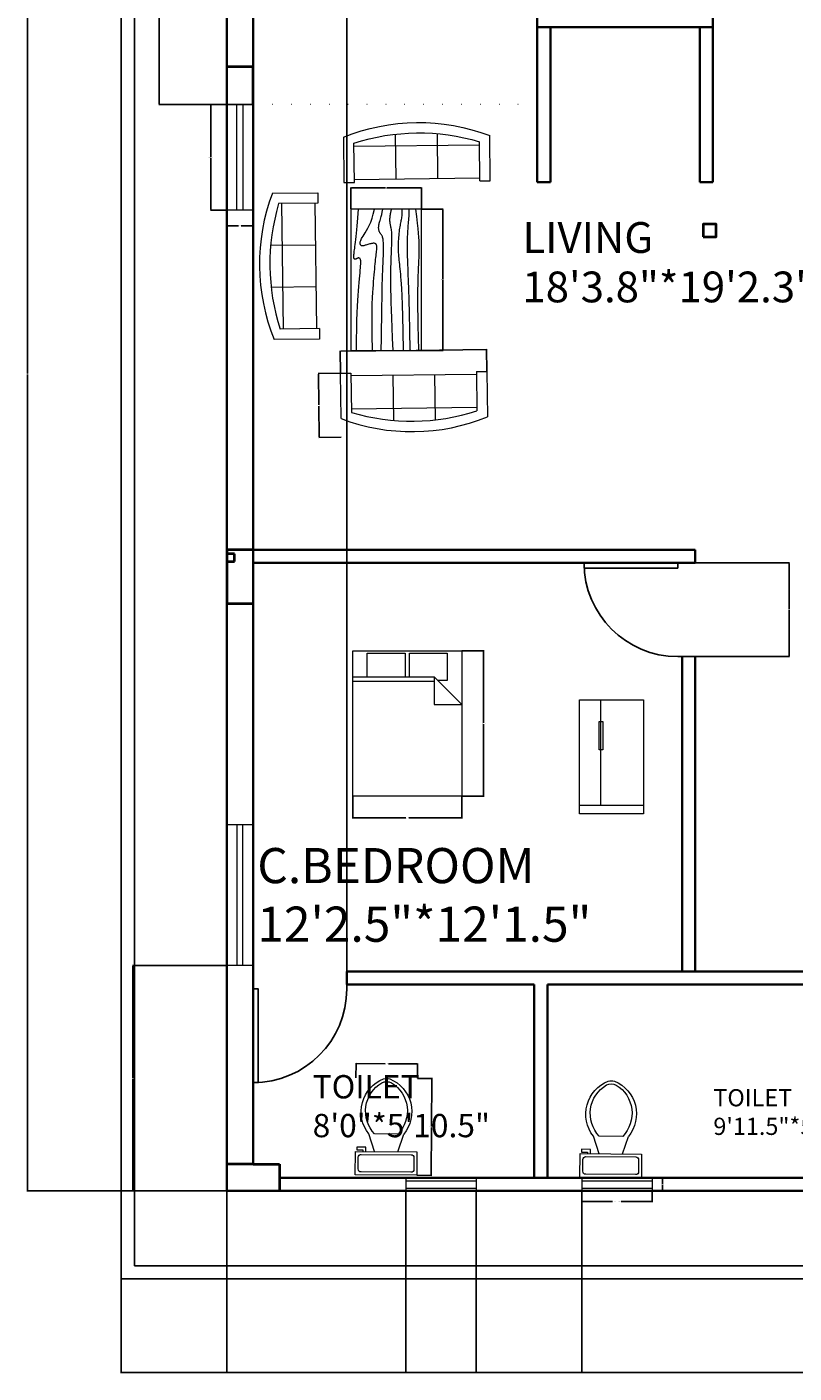
# Model space of a CAD drawing. Units: inches. Extents: x -1085 to 1941, y 1514 to 2348.
# Tile 7 of 9: x 1397 to 1659, y 1514 to 1974. Entities that reach past the tile are written whole.
import ezdxf

# ---------------------------------------------------------------- set-up
doc = ezdxf.new("R2010")
doc.units = ezdxf.units.IN
doc.linetypes.add('DOT', pattern=[6.35, 0, -6.35])
for name, color, linetype, lineweight in [('A-ANNO-DIMS', 2, 'Continuous', 18), ('A-AREA-IDEN', 7, 'Continuous', 25), ('A-COLS', 7, 'Continuous', 40), ('A-DOOR', 4, 'Continuous', 25), ('A-EQPM', 9, 'Continuous', 18), ('A-FLOR-FIXT', 9, 'Continuous', 18), ('A-GLAZ', 180, 'Continuous', 18), ('A-WALL', 7, 'Continuous', 35), ('A-WALL-OVHD', 8, 'DOT', 18), ('C-PROP', 8, 'Continuous', 25), ('FOUNITR-URE', 2, 'Continuous', 18)]:
    doc.layers.add(name, color=color, linetype=linetype, lineweight=lineweight)
doc.styles.get("Standard").update_dxf_attribs({"font": 'arial.ttf'})
doc.dimstyles.get("Standard").update_dxf_attribs({"dimtxt": 0.18, "dimasz": 0.18, "dimexe": 0.18, "dimexo": 0.0625, "dimgap": 0.09, "dimtad": 0, "dimtih": 1, "dimtoh": 1, "dimdec": 4, "dimzin": 0, "dimdsep": 46, "dimtxsty": 'Standard', "dimcen": 0.09, "dimadec": 0, "dimazin": 0, "dimtfac": 1, "dimtdec": 4, "dimtofl": 0, "dimtmove": 0, "dimatfit": 3, "dimfxl": 1, "dimtolj": 1, "dimtzin": 0, "dimarcsym": 0})

# ---------------------------------------------------------------- blocks, each defined once
blk = doc.blocks.new('*U3')
for p, q in [((0, 0), (0, -6)), ((32, 0), (32, -6))]:
    blk.add_line(p, q)
blk.add_lwpolyline([(0, 0), (0, 32), (1.75, 32), (1.75, 0)], close=True)
blk.add_arc((0, 0), 32, 0, 90)
blk = doc.blocks.new('Bed - Queen')
for p, q in [((0, -80.00003), (0, 0)), ((0, 0), (59.99999, 0)), ((59.99999, 0), (59.99999, -80.00003)), ((7.99999, -1.2), (28.79998, -1.2)), ((7.99999, -14.4), (7.99999, -1.2)), ((28.79998, -1.2), (28.79998, -14.4)), ((31.19999, -1.2), (51.99999, -1.2)), ((31.19999, -14.4), (31.19999, -1.2)), ((51.99999, -1.2), (51.99999, -16.4)), ((0, -14.4), (44.8, -14.4)), ((59.99999, -29.6), (44.8, -14.4)), ((44.8, -14.4), (44.8, -29.6)), ((44.8, -16.8), (0, -16.8)), ((51.99999, -16.4), (46.79936, -16.4)), ((44.8, -29.6), (59.99999, -29.6)), ((59.99999, -80.00003), (0, -80.00003))]:
    blk.add_line(p, q)
blk = doc.blocks.new('Refrigerator-2 door - 36 in front')
for p, q in [((12, 5), (12, 64)), ((0, 5), (36, 5))]:
    blk.add_line(p, q)
for points in [[(0, 0), (0, 64), (36, 64), (36, 0)], [(11, 36), (11, 52), (13, 52), (13, 36)]]:
    blk.add_lwpolyline(points, close=True)
blk = doc.blocks.new('Toilet - top')
for p, q in [((9.5, -6), (9.5, -2)), ((-10, -8.5), (-8, -8.5)), ((-10, -9.5), (-10, -8.5)), ((-8, -8.5), (-8, -8)), ((-7, -8), (-7, -9.5)), ((-4, -8), (-6, -14)), ((4, -8), (6, -14)), ((-7, -9.5), (-10, -9.5)), ((4, -14), (-4, -14))]:
    blk.add_line(p, q)
blk.add_lwpolyline([(10.5, -8), (10.5, 0), (-10.5, 0), (-10.5, -8)], close=True)
for points in [[(-9.5, -2), (-9.5, -6)], [(8.5, -1), (-8.5, -1)], [(-8.5, -7), (8.5, -7)]]:
    blk.add_lwpolyline(points)
for centre, radius, start, end in [((-8.62, -1.88), 0.884, 81.8699, 188.1301), ((8.62, -1.88), 0.884, 351.8699, 98.1301), ((-8.62, -6.12), 0.884, 171.8699, 278.1301), ((8.62, -6.12), 0.884, 261.8699, 8.1301), ((3.52, -21.58), 12.17, 141.4691, 247.9714), ((4.2, -21.82), 11.33, 136.3677, 238.9468), ((-3.52, -21.58), 12.17, 292.0284, 38.5307), ((-4.2, -21.82), 11.33, 301.053, 43.6321), ((0, -27.88), 4, 245.7318, 294.2682), ((0, -29), 4, 254.8605, 285.1395)]:
    blk.add_arc(centre, radius, start, end)
blk = doc.blocks.new('Table - Rectangular Woodgrain 60 x 30 in.')
for p, q in [((0, 0), (0, -30)), ((60, 0), (0, 0)), ((60, -30), (60, 0)), ((0, -30), (60, -30))]:
    blk.add_line(p, q)
for points in [[(0, -2.4), (4.8155, -2.418), (9.0302, -2.4688), (12.709, -2.5477), (15.9167, -2.65), (18.7181, -2.7711), (21.1781, -2.9063), (23.3616, -3.0508), (25.3333, -3.2), (27.1477, -3.3495), (28.8172, -3.4958), (30.3437, -3.636), (31.7291, -3.7667), (32.9756, -3.8849), (34.0849, -3.9875), (35.059, -4.0714), (35.9, -4.1334), (36.6114, -4.1711), (37.2041, -4.1854), (37.6906, -4.1779), (38.0833, -4.15), (38.3948, -4.1034), (38.6375, -4.0396), (38.8239, -3.9602), (38.9666, -3.8667), (39.0764, -3.7608), (39.1573, -3.6448), (39.2116, -3.521), (39.2416, -3.3917), (39.2498, -3.2593), (39.2385, -3.1261), (39.21, -2.9944), (39.1666, -2.8667), (39.111, -2.7447), (39.0468, -2.6281), (38.978, -2.5163), (38.9083, -2.4083), (38.8418, -2.3035), (38.7823, -2.201), (38.7337, -2.1001), (38.7, -2), (38.6844, -1.9003), (38.6875, -1.8021), (38.7094, -1.707), (38.75, -1.6167), (38.8094, -1.5326), (38.8875, -1.4563), (38.9844, -1.3893), (39.1, -1.3333), (39.2351, -1.2896), (39.3937, -1.2583), (39.5804, -1.2396), (39.8, -1.2333), (40.057, -1.2396), (40.3562, -1.2583), (40.7023, -1.2896), (41.1, -1.3333), (41.5547, -1.3895), (42.0755, -1.4573), (42.6721, -1.5361), (43.3542, -1.625), (44.1316, -1.7233), (45.014, -1.8302), (46.0114, -1.9449), (47.1333, -2.0667), (48.3862, -2.1947), (49.7625, -2.3281), (51.2513, -2.4663), (52.8416, -2.6083), (54.5226, -2.7535), (56.2833, -2.9011), (58.1127, -3.0501), (60, -3.2)], [(0, -9.2), (6.5759, -9.0858), (11.9385, -9.0365), (16.2527, -9.0418), (19.6833, -9.0917), (22.3952, -9.1759), (24.5531, -9.2844), (26.322, -9.4069), (27.8666, -9.5333), (29.3241, -9.6553), (30.7203, -9.7719), (32.0532, -9.8837), (33.3208, -9.9917), (34.5213, -10.0965), (35.6526, -10.199), (36.7128, -10.2999), (37.7, -10.4), (38.6129, -10.4996), (39.4531, -10.5969), (40.223, -10.6895), (40.925, -10.775), (41.5613, -10.8512), (42.1344, -10.9156), (42.6465, -10.966), (43.1, -11), (43.4976, -11.0158), (43.8437, -11.0136), (44.143, -10.9942), (44.4, -10.9583), (44.6195, -10.9069), (44.8062, -10.8406), (44.9648, -10.7603), (45.1, -10.6667), (45.2155, -10.5598), (45.3114, -10.4365), (45.3871, -10.2929), (45.4416, -10.125), (45.4743, -9.929), (45.4844, -9.7011), (45.4709, -9.4371), (45.4333, -9.1333), (45.3716, -8.7883), (45.2896, -8.4104), (45.1919, -8.0107), (45.0833, -7.6), (44.9685, -7.1893), (44.8521, -6.7896), (44.7388, -6.4117), (44.6333, -6.0667), (44.54, -5.7628), (44.4614, -5.4979), (44.4001, -5.2675), (44.3583, -5.0667), (44.3384, -4.8909), (44.3427, -4.7354), (44.3736, -4.5956), (44.4333, -4.4667), (44.5236, -4.3453), (44.6427, -4.2333), (44.7884, -4.1339), (44.9583, -4.05), (45.1501, -3.9849), (45.3614, -3.9417), (45.59, -3.9234), (45.8333, -3.9333), (46.0915, -3.9749), (46.3734, -4.0531), (46.6906, -4.1736), (47.0542, -4.3417), (47.4756, -4.5629), (47.9661, -4.8427), (48.5372, -5.1866), (49.2, -5.6), (49.9676, -6.0844), (50.8594, -6.625), (51.8965, -7.2031), (53.1, -7.8), (54.491, -8.3969), (56.0906, -8.975), (57.9199, -9.5156), (60, -10)], [(0, -12.8), (5.1847, -12.9322), (9.6213, -13.0323), (13.3963, -13.1059), (16.5958, -13.1583), (19.3063, -13.1952), (21.614, -13.2219), (23.6054, -13.2439), (25.3666, -13.2667), (26.9728, -13.2947), (28.4531, -13.3281), (29.8256, -13.3663), (31.1083, -13.4083), (32.3191, -13.4535), (33.476, -13.501), (34.597, -13.5501), (35.7, -13.6), (36.7984, -13.6497), (37.8875, -13.6979), (38.9578, -13.743), (40, -13.7833), (41.0047, -13.8174), (41.9625, -13.8438), (42.864, -13.8607), (43.7, -13.8667), (44.4631, -13.8604), (45.1552, -13.8417), (45.7801, -13.8104), (46.3416, -13.7667), (46.8439, -13.7104), (47.2906, -13.6417), (47.6858, -13.5604), (48.0333, -13.4667), (48.3375, -13.3608), (48.6042, -13.2448), (48.8396, -13.121), (49.05, -12.9917), (49.2417, -12.8593), (49.4208, -12.7261), (49.5937, -12.5944), (49.7667, -12.4667), (49.9452, -12.3451), (50.1323, -12.2313), (50.3303, -12.1268), (50.5416, -12.0333), (50.7686, -11.9524), (51.0135, -11.8854), (51.2788, -11.8341), (51.5666, -11.8), (51.8785, -11.7843), (52.2116, -11.7865), (52.562, -11.8059), (52.926, -11.8417), (53.2998, -11.8931), (53.6795, -11.9594), (54.0614, -12.0397), (54.4416, -12.1333), (54.8223, -12.2401), (55.2293, -12.3625), (55.6942, -12.5037), (56.2489, -12.6667), (56.9251, -12.8547), (57.7545, -13.0708), (58.7689, -13.3182), (60, -13.6)], [(0, -18), (5.124, -17.7273), (9.6609, -17.5057), (13.6705, -17.3303), (17.2125, -17.1958), (20.3467, -17.0973), (23.1328, -17.0297), (25.6307, -16.9878), (27.9, -16.9667), (29.9928, -16.9617), (31.9302, -16.9703), (33.7254, -16.9907), (35.3917, -17.0208), (36.9423, -17.0588), (38.3906, -17.1026), (39.7499, -17.1503), (41.0333, -17.2), (42.2519, -17.2496), (43.4073, -17.2969), (44.4986, -17.3395), (45.525, -17.375), (46.4858, -17.4012), (47.3802, -17.4156), (48.2074, -17.416), (48.9667, -17.4), (49.6583, -17.3662), (50.2872, -17.3167), (50.8595, -17.2547), (51.3812, -17.1833), (51.8584, -17.1057), (52.2971, -17.025), (52.7034, -16.9443), (53.0833, -16.8667), (53.443, -16.7951), (53.789, -16.7313), (54.128, -16.6768), (54.4666, -16.6334), (54.8115, -16.6024), (55.1693, -16.5854), (55.5465, -16.5841), (55.95, -16.6), (56.3828, -16.6337), (56.8346, -16.6823), (57.2915, -16.7418), (57.7396, -16.8084), (58.165, -16.878), (58.5539, -16.9469), (58.8924, -17.0111), (59.1666, -17.0667), (59.3679, -17.1107), (59.5078, -17.1438), (59.6032, -17.1675), (59.6708, -17.1833), (59.7275, -17.193), (59.7901, -17.1979), (59.8753, -17.1998), (60, -17.2)], [(0, -22.4), (8.0098, -22.2501), (14.4094, -22.1011), (19.4168, -21.9535), (23.25, -21.8083), (26.1269, -21.6663), (28.2656, -21.5281), (29.884, -21.3947), (31.2, -21.2667), (32.3967, -21.1448), (33.5172, -21.0292), (34.5697, -20.9198), (35.5625, -20.8167), (36.5037, -20.7198), (37.4015, -20.6292), (38.2642, -20.5448), (39.1, -20.4667), (39.9164, -20.3951), (40.7187, -20.3313), (41.5117, -20.2768), (42.3, -20.2333), (43.0883, -20.2024), (43.8812, -20.1854), (44.6836, -20.1841), (45.5, -20.2), (46.3328, -20.234), (47.1747, -20.2844), (48.0163, -20.3488), (48.8479, -20.425), (49.66, -20.5106), (50.4429, -20.6031), (51.1872, -20.7004), (51.8833, -20.8), (52.5246, -20.8999), (53.1166, -20.9995), (53.6681, -21.0983), (54.1875, -21.1958), (54.6834, -21.2919), (55.1646, -21.3859), (55.6394, -21.4777), (56.1167, -21.5667), (56.6028, -21.6515), (57.0961, -21.7266), (57.5929, -21.7852), (58.0896, -21.8208), (58.5823, -21.8268), (59.0674, -21.7964), (59.5412, -21.723), (60, -21.6)], [(0, -25.2), (8.6355, -25.0504), (15.7026, -24.9031), (21.4049, -24.7606), (25.9458, -24.625), (29.529, -24.4988), (32.3578, -24.3844), (34.6359, -24.284), (36.5667, -24.2), (38.3213, -24.1341), (39.9417, -24.0854), (41.437, -24.0523), (42.8167, -24.0333), (44.0901, -24.0268), (45.2667, -24.0313), (46.3557, -24.0451), (47.3667, -24.0667), (48.309, -24.0947), (49.1928, -24.1287), (50.0284, -24.168), (50.826, -24.2125), (51.5959, -24.2617), (52.3483, -24.3151), (53.0935, -24.3725), (53.8417, -24.4334), (54.6009, -24.497), (55.3699, -24.561), (56.1454, -24.6226), (56.9239, -24.6792), (57.7021, -24.7279), (58.4764, -24.7662), (59.2435, -24.7911), (60, -24.8)], [(0, -28.8), (5.6867, -28.6681), (10.45, -28.5698), (14.407, -28.5012), (17.675, -28.4584), (20.3711, -28.4374), (22.6125, -28.4344), (24.5164, -28.4455), (26.2, -28.4667), (27.762, -28.4947), (29.2276, -28.5281), (30.6033, -28.5663), (31.8958, -28.6084), (33.1118, -28.6535), (34.2578, -28.7011), (35.3405, -28.7501), (36.3666, -28.8), (37.3443, -28.8497), (38.288, -28.8974), (39.2137, -28.9412), (40.1375, -28.9792), (41.0753, -29.0093), (42.0432, -29.0297), (43.0572, -29.0384), (44.1333, -29.0333), (45.2936, -29.0114), (46.5843, -28.9641), (48.0579, -28.8816), (49.7666, -28.7542), (51.7629, -28.5721), (54.0989, -28.3255), (56.8272, -28.0048), (60, -27.6)]]:
    blk.add_lwpolyline(points)
blk = doc.blocks.new('Sofa - Roundback 7 ft.')
for p, q in [((-12.00002, -32.4421), (-12.00003, -6.5971)), ((11.99997, -32.4421), (11.99998, -6.5971)), ((-36.000027, -34), (-36.000027, -11.4696)), ((-35.999844, -13.3819), (35.9998, -13.3819)), ((35.99998, -34), (35.99998, -11.4696)), ((-36.000027, -32.4421), (35.99998, -32.4421))]:
    blk.add_line(p, q)
for points in [[(-36.000027, -34), (-42.000027, -34), (-42.000027, -8)], [(41.99998, -8), (41.99998, -34), (35.99998, -34)]]:
    blk.add_lwpolyline(points)
for centre, radius, start, end in [((0, -114.25), 114.25, 68.43141, 111.5686), ((-0.00001, -127.1968), 121.1968, 72.72033, 107.2797)]:
    blk.add_arc(centre, radius, start, end)
blk = doc.blocks.new('WIN-24-4.5')
for p, q in [((0, 4.5), (0, 0)), ((0, 3.5), (24, 3.5)), ((0, 1), (24, 1)), ((24, 4.5), (24, 0))]:
    blk.add_line(p, q)
blk = doc.blocks.new('WIN-36-9')
for p, q in [((0, 9), (0, 0)), ((0, 5.5), (36, 5.5)), ((36, 9), (36, 0)), ((36, 3.5), (0, 3.5))]:
    blk.add_line(p, q)
blk = doc.blocks.new('WIN-48-9')
for p, q in [((9, 48), (0, 48)), ((3.5, 48), (3.5, 0)), ((5.5, 0), (5.5, 48)), ((9, 0), (0, 0))]:
    blk.add_line(p, q)
blk = doc.blocks.new('*D34')
at = {"layer": 'A-ANNO-DIMS', "color": 0, "lineweight": -2, "transparency": 16777216}
for p, q in [((1545.41, 1760.71), (1552.97, 1760.71)), ((1552.79, 1760.53), (1552.79, 1736.08)), ((1552.79, 1711.27), (1552.79, 1735.72)), ((1545.41, 1711.09), (1552.97, 1711.09))]:
    blk.add_line(p, q, dxfattribs=at)
at = {"layer": 'A-ANNO-DIMS', "color": 0, "transparency": 16777216}
for points in [[(1552.76, 1760.53), (1552.82, 1760.53), (1552.79, 1760.71)], [(1552.76, 1711.27), (1552.82, 1711.27), (1552.79, 1711.09)]]:
    blk.add_solid(points, dxfattribs=at)
at = {"layer": 'Defpoints', "color": 0, "transparency": 16777216}
for p in [(1545.35, 1760.71), (1552.79, 1760.71), (1545.35, 1711.09)]:
    blk.add_point(p, dxfattribs=at)
at = {"layer": 'A-ANNO-DIMS', "color": 0, "transparency": 16777216, "insert": (1552.79, 1735.9), "char_height": 0.18, "attachment_point": 5}
blk.add_mtext('\\A1;BED 50 TYP.', dxfattribs=at)
blk = doc.blocks.new('*D35')
at = {"layer": 'A-ANNO-DIMS', "color": 0, "lineweight": -2, "transparency": 16777216}
for p, q in [((1508.14, 1711.03), (1508.14, 1703.47)), ((1545.35, 1711.03), (1545.35, 1703.47)), ((1508.32, 1703.65), (1526.21, 1703.65)), ((1545.17, 1703.65), (1527.27, 1703.65))]:
    blk.add_line(p, q, dxfattribs=at)
at = {"layer": 'A-ANNO-DIMS', "color": 0, "transparency": 16777216}
for points in [[(1508.32, 1703.68), (1508.32, 1703.62), (1508.14, 1703.65)], [(1545.17, 1703.68), (1545.17, 1703.62), (1545.35, 1703.65)]]:
    blk.add_solid(points, dxfattribs=at)
at = {"layer": 'Defpoints', "color": 0, "transparency": 16777216}
for p in [(1508.14, 1711.09), (1545.35, 1711.09), (1545.35, 1703.65)]:
    blk.add_point(p, dxfattribs=at)
at = {"layer": 'A-ANNO-DIMS', "color": 0, "transparency": 16777216, "insert": (1526.74, 1703.65), "char_height": 0.18, "attachment_point": 5}
blk.add_mtext('\\A1;37 TYP.', dxfattribs=at)
blk = doc.blocks.new('*D40')
at = {"layer": 'A-ANNO-DIMS', "color": 0, "lineweight": -2, "transparency": 16777216}
for p, q in [((1503.95, 1855.55), (1503.85, 1863.17)), ((1504.04, 1862.99), (1527.94, 1863.28)), ((1553.66, 1863.6), (1529.75, 1863.3)), ((1553.93, 1856.16), (1553.84, 1863.78))]:
    blk.add_line(p, q, dxfattribs=at)
at = {"layer": 'A-ANNO-DIMS', "color": 0, "transparency": 16777216}
for points in [[(1504.03, 1863.02), (1504.04, 1862.96), (1503.86, 1862.99)], [(1553.66, 1863.63), (1553.66, 1863.57), (1553.84, 1863.6)]]:
    blk.add_solid(points, dxfattribs=at)
at = {"layer": 'Defpoints', "color": 0, "transparency": 16777216}
for p in [(1503.86, 1862.99), (1503.95, 1855.49), (1553.93, 1856.1)]:
    blk.add_point(p, dxfattribs=at)
at = {"layer": 'A-ANNO-DIMS', "color": 0, "transparency": 16777216, "insert": (1528.85, 1863.29), "char_height": 0.18, "attachment_point": 5}
blk.add_mtext('\\A1;SOFA 50 TYP.', dxfattribs=at)
blk = doc.blocks.new('*D41')
at = {"layer": 'A-ANNO-DIMS', "color": 0, "lineweight": -2, "transparency": 16777216}
for p, q in [((1503.88, 1855.49), (1496.27, 1855.39)), ((1496.45, 1855.22), (1496.58, 1844.67)), ((1496.71, 1833.76), (1496.59, 1844.31)), ((1504.15, 1833.67), (1496.54, 1833.58))]:
    blk.add_line(p, q, dxfattribs=at)
at = {"layer": 'A-ANNO-DIMS', "color": 0, "transparency": 16777216}
for points in [[(1496.48, 1855.22), (1496.42, 1855.22), (1496.45, 1855.4)], [(1496.74, 1833.76), (1496.68, 1833.76), (1496.72, 1833.58)]]:
    blk.add_solid(points, dxfattribs=at)
at = {"layer": 'Defpoints', "color": 0, "transparency": 16777216}
for p in [(1503.95, 1855.49), (1496.72, 1833.58), (1504.21, 1833.67)]:
    blk.add_point(p, dxfattribs=at)
at = {"layer": 'A-ANNO-DIMS', "color": 0, "transparency": 16777216, "insert": (1496.58, 1844.49), "char_height": 0.18, "attachment_point": 5}
blk.add_mtext('\\A1;22 TYP.', dxfattribs=at)
blk = doc.blocks.new('*D46')
at = {"layer": 'A-ANNO-DIMS', "color": 0, "lineweight": -2, "transparency": 16777216}
for p, q in [((1531.69, 1911.56), (1539.04, 1911.56)), ((1538.86, 1911.38), (1538.86, 1887.61)), ((1538.86, 1863.49), (1538.86, 1887.25)), ((1531.69, 1863.31), (1539.04, 1863.31))]:
    blk.add_line(p, q, dxfattribs=at)
at = {"layer": 'A-ANNO-DIMS', "color": 0, "transparency": 16777216}
for points in [[(1538.83, 1911.38), (1538.89, 1911.38), (1538.86, 1911.56)], [(1538.83, 1863.49), (1538.89, 1863.49), (1538.86, 1863.31)]]:
    blk.add_solid(points, dxfattribs=at)
at = {"layer": 'Defpoints', "color": 0, "transparency": 16777216}
for p in [(1531.62, 1911.56), (1538.86, 1911.56), (1531.62, 1863.31)]:
    blk.add_point(p, dxfattribs=at)
at = {"layer": 'A-ANNO-DIMS', "color": 0, "transparency": 16777216, "insert": (1538.86, 1887.43), "char_height": 0.18, "attachment_point": 5}
blk.add_mtext('\\A1;TABLE 48', dxfattribs=at)
blk = doc.blocks.new('*D47')
at = {"layer": 'A-ANNO-DIMS', "color": 0, "lineweight": -2, "transparency": 16777216}
for p, q in [((1507.5, 1911.62), (1507.5, 1918.97)), ((1507.68, 1918.79), (1519.34, 1918.79)), ((1531.44, 1918.79), (1519.78, 1918.79)), ((1531.62, 1911.62), (1531.62, 1918.97))]:
    blk.add_line(p, q, dxfattribs=at)
at = {"layer": 'A-ANNO-DIMS', "color": 0, "transparency": 16777216}
for points in [[(1507.68, 1918.82), (1507.68, 1918.76), (1507.5, 1918.79)], [(1531.44, 1918.82), (1531.44, 1918.76), (1531.62, 1918.79)]]:
    blk.add_solid(points, dxfattribs=at)
at = {"layer": 'Defpoints', "color": 0, "transparency": 16777216}
for p in [(1507.5, 1918.79), (1507.5, 1911.56), (1531.62, 1911.56)]:
    blk.add_point(p, dxfattribs=at)
at = {"layer": 'A-ANNO-DIMS', "color": 0, "transparency": 16777216, "insert": (1519.56, 1918.79), "char_height": 0.18, "attachment_point": 5}
blk.add_mtext('\\A1;24', dxfattribs=at)
blk = doc.blocks.new('*D60')
at = {"layer": 'A-ANNO-DIMS', "color": 0, "lineweight": -2, "transparency": 16777216}
for p, q in [((1530.28, 1614.66), (1535.36, 1614.62)), ((1535.18, 1614.44), (1535.06, 1598.28)), ((1534.95, 1581.76), (1535.06, 1597.92)), ((1530.05, 1581.61), (1535.12, 1581.57))]:
    blk.add_line(p, q, dxfattribs=at)
at = {"layer": 'A-ANNO-DIMS', "color": 0, "transparency": 16777216}
for points in [[(1535.15, 1614.44), (1535.21, 1614.44), (1535.18, 1614.62)], [(1534.92, 1581.76), (1534.98, 1581.76), (1534.94, 1581.58)]]:
    blk.add_solid(points, dxfattribs=at)
at = {"layer": 'Defpoints', "color": 0, "transparency": 16777216}
for p in [(1530.22, 1614.66), (1529.99, 1581.61), (1534.94, 1581.58)]:
    blk.add_point(p, dxfattribs=at)
at = {"layer": 'A-ANNO-DIMS', "color": 0, "transparency": 16777216, "insert": (1535.06, 1598.1), "char_height": 0.18, "attachment_point": 5}
blk.add_mtext('\\A1;WC 33 TYP.', dxfattribs=at)
blk = doc.blocks.new('*D61')
at = {"layer": 'A-ANNO-DIMS', "color": 0, "lineweight": -2, "transparency": 16777216}
for p, q in [((1509.22, 1614.87), (1509.26, 1619.94)), ((1509.44, 1619.76), (1519.23, 1619.69)), ((1530.08, 1619.61), (1520.29, 1619.68)), ((1530.22, 1614.72), (1530.26, 1619.79))]:
    blk.add_line(p, q, dxfattribs=at)
at = {"layer": 'A-ANNO-DIMS', "color": 0, "transparency": 16777216}
for points in [[(1509.44, 1619.79), (1509.44, 1619.73), (1509.26, 1619.76)], [(1530.08, 1619.64), (1530.08, 1619.58), (1530.26, 1619.61)]]:
    blk.add_solid(points, dxfattribs=at)
at = {"layer": 'Defpoints', "color": 0, "transparency": 16777216}
for p in [(1530.26, 1619.61), (1509.22, 1614.81), (1530.22, 1614.66)]:
    blk.add_point(p, dxfattribs=at)
at = {"layer": 'A-ANNO-DIMS', "color": 0, "transparency": 16777216, "insert": (1519.76, 1619.69), "char_height": 0.18, "attachment_point": 5}
blk.add_mtext('\\A1;21 TYP.', dxfattribs=at)
blk = doc.blocks.new('*D64')
at = {"layer": 'A-ANNO-DIMS', "color": 0, "lineweight": -2, "transparency": 16777216}
for p, q in [((1586.33, 1576.18), (1586.33, 1572.46)), ((1586.51, 1572.64), (1596.85, 1572.64)), ((1610.15, 1572.64), (1599.81, 1572.64)), ((1610.33, 1576.18), (1610.33, 1572.46))]:
    blk.add_line(p, q, dxfattribs=at)
at = {"layer": 'A-ANNO-DIMS', "color": 0, "transparency": 16777216}
for points in [[(1586.51, 1572.67), (1586.51, 1572.61), (1586.33, 1572.64)], [(1610.15, 1572.67), (1610.15, 1572.61), (1610.33, 1572.64)]]:
    blk.add_solid(points, dxfattribs=at)
at = {"layer": 'Defpoints', "color": 0, "transparency": 16777216}
for p in [(1586.33, 1576.24), (1610.33, 1576.24), (1610.33, 1572.64)]:
    blk.add_point(p, dxfattribs=at)
at = {"layer": 'A-ANNO-DIMS', "color": 0, "transparency": 16777216, "insert": (1598.33, 1572.64), "char_height": 0.18, "attachment_point": 5}
blk.add_mtext('\\A1;BATH WINDOW 24 TYP.', dxfattribs=at)
blk = doc.blocks.new('*D65')
at = {"layer": 'A-ANNO-DIMS', "color": 0, "lineweight": -2, "transparency": 16777216}
for p, q in [((1610.39, 1580.74), (1614.11, 1580.74)), ((1613.93, 1580.56), (1613.93, 1578.67)), ((1613.93, 1576.42), (1613.93, 1578.31)), ((1610.39, 1576.24), (1614.11, 1576.24))]:
    blk.add_line(p, q, dxfattribs=at)
at = {"layer": 'A-ANNO-DIMS', "color": 0, "transparency": 16777216}
for points in [[(1613.9, 1580.56), (1613.96, 1580.56), (1613.93, 1580.74)], [(1613.9, 1576.42), (1613.96, 1576.42), (1613.93, 1576.24)]]:
    blk.add_solid(points, dxfattribs=at)
at = {"layer": 'Defpoints', "color": 0, "transparency": 16777216}
for p in [(1610.33, 1580.74), (1613.93, 1580.74), (1610.33, 1576.24)]:
    blk.add_point(p, dxfattribs=at)
at = {"layer": 'A-ANNO-DIMS', "color": 0, "transparency": 16777216, "insert": (1613.93, 1578.49), "char_height": 0.18, "attachment_point": 5}
blk.add_mtext('\\A1;5 TYP.', dxfattribs=at)
blk = doc.blocks.new('*D66')
at = {"layer": 'A-ANNO-DIMS', "color": 0, "lineweight": -2, "transparency": 16777216}
for p, q in [((1465.03, 1947.24), (1459.51, 1947.24)), ((1459.69, 1947.06), (1459.69, 1929.42)), ((1459.69, 1911.42), (1459.69, 1929.06)), ((1465.03, 1911.24), (1459.51, 1911.24))]:
    blk.add_line(p, q, dxfattribs=at)
at = {"layer": 'A-ANNO-DIMS', "color": 0, "transparency": 16777216}
for points in [[(1459.66, 1947.06), (1459.72, 1947.06), (1459.69, 1947.24)], [(1459.66, 1911.42), (1459.72, 1911.42), (1459.69, 1911.24)]]:
    blk.add_solid(points, dxfattribs=at)
at = {"layer": 'Defpoints', "color": 0, "transparency": 16777216}
for p in [(1465.09, 1947.24), (1459.69, 1911.24), (1465.09, 1911.24)]:
    blk.add_point(p, dxfattribs=at)
at = {"layer": 'A-ANNO-DIMS', "color": 0, "transparency": 16777216, "insert": (1459.69, 1929.24), "char_height": 0.18, "attachment_point": 5}
blk.add_mtext('\\A1;WINDOW 36 TYP.', dxfattribs=at)
blk = doc.blocks.new('*D67')
at = {"layer": 'A-ANNO-DIMS', "color": 0, "lineweight": -2, "transparency": 16777216}
for p, q in [((1465.09, 1911.18), (1465.09, 1905.66)), ((1474.09, 1911.18), (1474.09, 1905.66)), ((1465.27, 1905.84), (1469.14, 1905.84)), ((1473.91, 1905.84), (1470.05, 1905.84))]:
    blk.add_line(p, q, dxfattribs=at)
at = {"layer": 'A-ANNO-DIMS', "color": 0, "transparency": 16777216}
for points in [[(1465.27, 1905.87), (1465.27, 1905.81), (1465.09, 1905.84)], [(1473.91, 1905.87), (1473.91, 1905.81), (1474.09, 1905.84)]]:
    blk.add_solid(points, dxfattribs=at)
at = {"layer": 'Defpoints', "color": 0, "transparency": 16777216}
for p in [(1465.09, 1911.24), (1474.09, 1911.24), (1474.09, 1905.84)]:
    blk.add_point(p, dxfattribs=at)
at = {"layer": 'A-ANNO-DIMS', "color": 0, "transparency": 16777216, "insert": (1469.59, 1905.84), "char_height": 0.18, "attachment_point": 5}
blk.add_mtext('\\A1;9 TYP.', dxfattribs=at)
blk = doc.blocks.new('*D74')
at = {"layer": 'A-ANNO-DIMS', "color": 0, "lineweight": -2, "transparency": 16777216}
for p, q in [((1429.09, 1546.18), (1429.09, 1514.06)), ((1909.09, 1546.18), (1909.09, 1514.06)), ((1429.27, 1514.24), (1668.8, 1514.24)), ((1908.91, 1514.24), (1669.39, 1514.24))]:
    blk.add_line(p, q, dxfattribs=at)
at = {"layer": 'A-ANNO-DIMS', "color": 0, "transparency": 16777216}
for points in [[(1429.27, 1514.27), (1429.27, 1514.21), (1429.09, 1514.24)], [(1908.91, 1514.27), (1908.91, 1514.21), (1909.09, 1514.24)]]:
    blk.add_solid(points, dxfattribs=at)
at = {"layer": 'Defpoints', "color": 0, "transparency": 16777216}
for p in [(1429.09, 1546.24), (1909.09, 1546.24), (1909.09, 1514.24)]:
    blk.add_point(p, dxfattribs=at)
at = {"layer": 'A-ANNO-DIMS', "color": 0, "transparency": 16777216, "insert": (1669.09, 1514.24), "char_height": 0.18, "attachment_point": 5}
blk.add_mtext('\\A1;480', dxfattribs=at)
blk = doc.blocks.new('*D77')
at = {"layer": 'A-ANNO-DIMS', "color": 0, "lineweight": -2, "transparency": 16777216}
for p, q in [((1465.03, 2134.24), (1396.91, 2134.24)), ((1397.09, 2134.06), (1397.09, 1855.42)), ((1397.09, 1576.42), (1397.09, 1855.06)), ((1465.03, 1576.24), (1396.91, 1576.24))]:
    blk.add_line(p, q, dxfattribs=at)
at = {"layer": 'A-ANNO-DIMS', "color": 0, "transparency": 16777216}
for points in [[(1397.06, 2134.06), (1397.12, 2134.06), (1397.09, 2134.24)], [(1397.06, 1576.42), (1397.12, 1576.42), (1397.09, 1576.24)]]:
    blk.add_solid(points, dxfattribs=at)
at = {"layer": 'Defpoints', "color": 0, "transparency": 16777216}
for p in [(1397.09, 2134.24), (1465.09, 2134.24), (1465.09, 1576.24)]:
    blk.add_point(p, dxfattribs=at)
at = {"layer": 'A-ANNO-DIMS', "color": 0, "transparency": 16777216, "insert": (1397.09, 1855.24), "char_height": 0.18, "attachment_point": 5}
blk.add_mtext('\\A1;558', dxfattribs=at)
blk = doc.blocks.new('*D83')
at = {"layer": 'A-ANNO-DIMS', "color": 0, "lineweight": -2, "transparency": 16777216}
for p, q in [((1625.16, 1790.74), (1657.27, 1790.74)), ((1657.09, 1790.56), (1657.09, 1774.92)), ((1657.09, 1758.92), (1657.09, 1774.56)), ((1625.16, 1758.74), (1657.27, 1758.74))]:
    blk.add_line(p, q, dxfattribs=at)
at = {"layer": 'A-ANNO-DIMS', "color": 0, "transparency": 16777216}
for points in [[(1657.06, 1790.56), (1657.12, 1790.56), (1657.09, 1790.74)], [(1657.06, 1758.92), (1657.12, 1758.92), (1657.09, 1758.74)]]:
    blk.add_solid(points, dxfattribs=at)
at = {"layer": 'Defpoints', "color": 0, "transparency": 16777216}
for p in [(1625.09, 1790.74), (1625.09, 1758.74), (1657.09, 1758.74)]:
    blk.add_point(p, dxfattribs=at)
at = {"layer": 'A-ANNO-DIMS', "color": 0, "transparency": 16777216, "insert": (1657.09, 1774.74), "char_height": 0.18, "attachment_point": 5}
blk.add_mtext('\\A1;32', dxfattribs=at)
blk = doc.blocks.new('*D84')
at = {"layer": 'A-ANNO-DIMS', "color": 0, "lineweight": -2, "transparency": 16777216}
for p, q in [((1474.09, 1651.3), (1474.09, 2214.42)), ((1474.27, 2214.24), (1489.88, 2214.24)), ((1505.91, 2214.24), (1490.31, 2214.24)), ((1506.09, 1651.3), (1506.09, 2214.42))]:
    blk.add_line(p, q, dxfattribs=at)
at = {"layer": 'A-ANNO-DIMS', "color": 0, "transparency": 16777216}
for points in [[(1474.27, 2214.27), (1474.27, 2214.21), (1474.09, 2214.24)], [(1505.91, 2214.27), (1505.91, 2214.21), (1506.09, 2214.24)]]:
    blk.add_solid(points, dxfattribs=at)
at = {"layer": 'Defpoints', "color": 0, "transparency": 16777216}
for p in [(1506.09, 2214.24), (1474.09, 1651.24), (1506.09, 1651.24)]:
    blk.add_point(p, dxfattribs=at)
at = {"layer": 'A-ANNO-DIMS', "color": 0, "transparency": 16777216, "insert": (1490.09, 2214.24), "char_height": 0.18, "attachment_point": 5}
blk.add_mtext('\\A1;32', dxfattribs=at)
blk = doc.blocks.new('*D86')
at = {"layer": 'A-ANNO-DIMS', "color": 0, "lineweight": -2, "transparency": 16777216}
for p, q in [((1465.09, 1576.18), (1465.09, 1514.06)), ((1526.28, 1576.18), (1526.28, 1514.06)), ((1465.27, 1514.24), (1495.29, 1514.24)), ((1526.1, 1514.24), (1496.08, 1514.24))]:
    blk.add_line(p, q, dxfattribs=at)
at = {"layer": 'A-ANNO-DIMS', "color": 0, "transparency": 16777216}
for points in [[(1465.27, 1514.27), (1465.27, 1514.21), (1465.09, 1514.24)], [(1526.1, 1514.27), (1526.1, 1514.21), (1526.28, 1514.24)]]:
    blk.add_solid(points, dxfattribs=at)
at = {"layer": 'Defpoints', "color": 0, "transparency": 16777216}
for p in [(1465.09, 1576.24), (1526.28, 1576.24), (1526.28, 1514.24)]:
    blk.add_point(p, dxfattribs=at)
at = {"layer": 'A-ANNO-DIMS', "color": 0, "transparency": 16777216, "insert": (1495.69, 1514.24), "char_height": 0.18, "attachment_point": 5}
blk.add_mtext('\\A1;61.19', dxfattribs=at)
blk = doc.blocks.new('*D87')
at = {"layer": 'A-ANNO-DIMS', "color": 0, "lineweight": -2, "transparency": 16777216}
for p, q in [((1550.28, 1576.18), (1550.28, 1514.06)), ((1586.33, 1576.18), (1586.33, 1514.06)), ((1550.46, 1514.24), (1567.84, 1514.24)), ((1586.15, 1514.24), (1568.77, 1514.24))]:
    blk.add_line(p, q, dxfattribs=at)
at = {"layer": 'A-ANNO-DIMS', "color": 0, "transparency": 16777216}
for points in [[(1550.46, 1514.27), (1550.46, 1514.21), (1550.28, 1514.24)], [(1586.15, 1514.27), (1586.15, 1514.21), (1586.33, 1514.24)]]:
    blk.add_solid(points, dxfattribs=at)
at = {"layer": 'Defpoints', "color": 0, "transparency": 16777216}
for p in [(1550.28, 1576.24), (1586.33, 1576.24), (1586.33, 1514.24)]:
    blk.add_point(p, dxfattribs=at)
at = {"layer": 'A-ANNO-DIMS', "color": 0, "transparency": 16777216, "insert": (1568.31, 1514.24), "char_height": 0.18, "attachment_point": 5}
blk.add_mtext('\\A1;36.046', dxfattribs=at)
blk = doc.blocks.new('*D89')
at = {"layer": 'A-ANNO-DIMS', "color": 0, "lineweight": -2, "transparency": 16777216}
for p, q in [((1465.03237, 1653.239219), (1432.91487, 1653.239219)), ((1433.09487, 1653.059219), (1433.09487, 1614.919219)), ((1433.09487, 1576.419219), (1433.09487, 1614.559219)), ((1465.03237, 1576.239219), (1432.91487, 1576.239219))]:
    blk.add_line(p, q, dxfattribs=at)
at = {"layer": 'A-ANNO-DIMS', "color": 0, "transparency": 16777216}
for points in [[(1433.06487, 1653.059219), (1433.12487, 1653.059219), (1433.09487, 1653.239219)], [(1433.06487, 1576.419219), (1433.12487, 1576.419219), (1433.09487, 1576.239219)]]:
    blk.add_solid(points, dxfattribs=at)
at = {"layer": 'Defpoints', "color": 0, "transparency": 16777216}
for p in [(1433.09487, 1653.239219), (1465.09487, 1653.239219), (1465.09487, 1576.239219)]:
    blk.add_point(p, dxfattribs=at)
at = {"layer": 'A-ANNO-DIMS', "color": 0, "transparency": 16777216, "insert": (1433.09487, 1614.739219), "char_height": 0.18, "attachment_point": 5}
blk.add_mtext('\\A1;77', dxfattribs=at)
blk = doc.blocks.new('*D90')
at = {"layer": 'A-ANNO-DIMS', "color": 0, "lineweight": -2, "transparency": 16777216}
for p, q in [((1474.03, 2045.74), (1441.91, 2045.74)), ((1442.09, 2045.56), (1442.09, 1996.67)), ((1442.09, 1947.42), (1442.09, 1996.31)), ((1474.03, 1947.24), (1441.91, 1947.24))]:
    blk.add_line(p, q, dxfattribs=at)
at = {"layer": 'A-ANNO-DIMS', "color": 0, "transparency": 16777216}
for points in [[(1442.06, 2045.56), (1442.12, 2045.56), (1442.09, 2045.74)], [(1442.06, 1947.42), (1442.12, 1947.42), (1442.09, 1947.24)]]:
    blk.add_solid(points, dxfattribs=at)
at = {"layer": 'Defpoints', "color": 0, "transparency": 16777216}
for p in [(1442.09, 2045.74), (1474.09, 2045.74), (1474.09, 1947.24)]:
    blk.add_point(p, dxfattribs=at)
at = {"layer": 'A-ANNO-DIMS', "color": 0, "transparency": 16777216, "insert": (1442.09, 1996.49), "char_height": 0.18, "attachment_point": 5}
blk.add_mtext('\\A1;98.5', dxfattribs=at)

msp = doc.modelspace()

# ---------------------------------------------------------------- linework, layer by layer
at = {"layer": 'A-COLS'}
for p, q in [((1474.0949, 1960.139), (1465.0949, 1960.139)), ((1474.0949, 1947.2392), (1474.0949, 1960.139)), ((1474.0949, 1795.2392), (1465.0949, 1795.2392)), ((1465.0949, 1795.2392), (1465.0949, 1776.8802)), ((1467.7837, 1793.8582), (1465.0949, 1793.8582)), ((1467.7837, 1791.2129), (1467.7837, 1793.8582)), ((1465.0949, 1791.2129), (1467.7837, 1791.2129)), ((1465.0949, 1776.8802), (1474.0949, 1776.8802)), ((1474.0949, 1585.4303), (1465.0949, 1585.4303)), ((1474.0949, 1585.4303), (1483.0949, 1585.4303)), ((1483.0949, 1585.4303), (1483.0949, 1576.2392))]:
    msp.add_line(p, q, dxfattribs=at)
msp.add_lwpolyline([(1627.8146, 1902.0881), (1632.1604, 1902.0881), (1632.1604, 1906.4629), (1627.8146, 1906.4629)], close=True, dxfattribs=at)
at = {"layer": 'A-GLAZ'}
for p, q in [((1465.0949, 1947.2392), (1474.0949, 1947.2392)), ((1474.0949, 1947.2392), (1474.0949, 1911.2392)), ((1474.0949, 1653.2392), (1474.0949, 1701.2392)), ((1526.2836, 1579.7392), (1550.2836, 1579.7392)), ((1526.2836, 1577.2392), (1550.2836, 1577.2392))]:
    msp.add_line(p, q, dxfattribs=at)
at = {"layer": 'A-WALL'}
for p, q in [((1465.0949, 2134.2392), (1465.0949, 1576.2392)), ((1474.0949, 2120.553), (1474.0949, 1585.4303)), ((1571.0949, 1973.7392), (1571.0949, 2036.7392)), ((1631.0949, 2036.7392), (1631.0949, 1973.7392)), ((1622.0949, 1973.7392), (1571.0949, 1973.7392)), ((1571.0949, 1973.7392), (1571.0949, 1920.7392)), ((1571.0949, 1973.7392), (1571.0949, 1944.7392)), ((1575.5949, 1973.7392), (1575.5949, 1920.7392)), ((1631.0949, 1973.7392), (1622.0949, 1973.7392)), ((1626.5949, 1973.7392), (1626.5949, 1920.7392)), ((1631.0949, 1973.7392), (1631.0949, 1920.7392)), ((1571.0949, 1920.7392), (1575.5949, 1920.7392)), ((1626.5949, 1920.7392), (1631.0949, 1920.7392)), ((1625.0949, 1795.2392), (1474.0949, 1795.2392)), ((1625.0949, 1790.7392), (1625.0949, 1795.2392)), ((1625.0949, 1790.7392), (1474.0949, 1790.7392)), ((1474.0949, 1651.2392), (1474.0949, 1759.2392)), ((1620.5949, 1651.2392), (1620.5949, 1758.7392)), ((1625.0949, 1651.2392), (1625.0949, 1758.7392)), ((1474.0949, 1585.4303), (1474.0949, 1676.7392)), ((1474.0949, 1651.2392), (1474.0949, 1653.2392)), ((1474.0949, 1585.4303), (1474.0949, 1651.2392)), ((1698.5949, 1651.2392), (1506.0949, 1651.2392)), ((1506.0949, 1646.7392), (1506.0949, 1651.2392)), ((1506.0949, 1651.2392), (1620.5949, 1651.2392)), ((1570.0949, 1646.7392), (1506.0949, 1646.7392)), ((1570.0949, 1580.7392), (1570.0949, 1646.7392)), ((1574.5949, 1580.7392), (1574.5949, 1646.7392)), ((1694.0949, 1646.7392), (1574.5949, 1646.7392)), ((1483.0949, 1580.7392), (1689.5637, 1580.7392)), ((1465.0949, 1576.2392), (1879.0949, 1576.2392))]:
    msp.add_line(p, q, dxfattribs=at)
at = {"layer": 'A-WALL-OVHD'}
msp.add_line((1571.0949, 1947.2392), (1474.0949, 1947.2392), dxfattribs=at)
at = {"layer": 'C-PROP'}
for p, q in [((1429.0949, 2182.2392), (1429.0949, 1546.2392)), ((1433.5949, 2177.7392), (1433.5949, 1550.7392)), ((1433.5949, 1550.7392), (1904.5949, 1550.7392)), ((1429.0949, 1546.2392), (1909.0949, 1546.2392))]:
    msp.add_line(p, q, dxfattribs=at)

# ---------------------------------------------------------------- block references
at = {"layer": 'A-DOOR', "xscale": -1}
for p, rotation in [((1619.0949, 1790.7392), 90), ((1474.0949, 1645.2392), 180)]:
    msp.add_blockref('*U3', p, dxfattribs=dict(at, rotation=rotation))
at = {"layer": 'A-EQPM', "xscale": 0.6082930186288423, "yscale": 0.6082930186288423, "zscale": 0.6082930186288423}
msp.add_blockref('Refrigerator-2 door - 36 in front', (1585.5575, 1704.9981), dxfattribs=at)
at = {"layer": 'A-FLOR-FIXT', "xscale": -1, "rotation": 179.5948752856431}
for p in [(1519.4872, 1581.6853), (1596.1931, 1580.9168)]:
    msp.add_blockref('Toilet - top', p, dxfattribs=at)
at = {"layer": 'A-GLAZ', "rotation": 270.0000000000009}
msp.add_blockref('WIN-36-9', (1465.0947, 1947.2391), dxfattribs=at)
at = {"layer": 'A-GLAZ'}
for name, p in [('WIN-48-9', (1465.095, 1653.239)), ('WIN-24-4.5', (1526.284, 1576.239)), ('WIN-24-4.5', (1586.3297, 1576.239))]:
    msp.add_blockref(name, p, dxfattribs=at)
at = {"layer": 'FOUNITR-URE'}
for name, p, xscale, yscale, zscale, rotation in [('Sofa - Roundback 7 ft.', (1529.8702, 1941.1465), -0.5951175733769987, 0.5951175733769988, 0.5951175733769988, 0.6524570325598323), ('Sofa - Roundback 7 ft.', (1476.2705, 1891.9176), 0.5951175733769988, 0.5951175733769988, 0.5951175733769988, 90.70274874306504), ('Table - Rectangular Woodgrain 60 x 30 in.', (1507.4991, 1863.3082), 0.8041531877972335, 0.8041531877972335, 0.8041531877972335, 90), ('Sofa - Roundback 7 ft.', (1529.1883, 1835.563), 0.5951175733769988, 0.5951175733769988, 0.5951175733769988, 180.7027487430649)]:
    msp.add_blockref(name, p, dxfattribs=dict(at, xscale=xscale, yscale=yscale, zscale=zscale, rotation=rotation))
at = {"layer": 'FOUNITR-URE', "xscale": 0.6202052364975769, "yscale": 0.6202052364975769, "zscale": 0.6202052364975769}
msp.add_blockref('Bed - Queen', (1508.136, 1760.7086), dxfattribs=at)

# ---------------------------------------------------------------- texts
at = {"layer": 'A-ANNO-DIMS'}
msp.add_text('18\'3.8"*19\'2.3"', height=10.510424, dxfattribs=at).set_placement((1566.056, 1879.7196))
at = {"layer": 'A-AREA-IDEN'}
msp.add_text('LIVING ', height=10.51042, dxfattribs=at).set_placement((1566.056, 1896.6037))
at = {"layer": 'A-AREA-IDEN', "attachment_point": 1}
for s, width, gutter_width, insert, char_height in [('C.BEDROOM\\P12\'2.5"*12\'1.5"', 6.473982, 60, (1475.5427, 1693.3645), 12), ('TOILET\\P8\'0"*5\'10.5"', 1.168897, 39.7844, (1494.4436, 1615.8213), 7.956871), ('TOILET\\P9\'11.5"*5\'10.5"', 0.197712, 29.3074, (1631.2558, 1611.0202), 5.861483)]:
    msp.add_mtext_dynamic_manual_height_columns(s, width=width, gutter_width=gutter_width, heights=[0], dxfattribs=dict(at, insert=insert, char_height=char_height))

# ---------------------------------------------------------------- dimensions: what is measured, and where the dimension line sits
at = {"layer": 'A-ANNO-DIMS'}
for base, p1, p2, override, picture, middle in [((1506.0949, 2214.2392), (1474.0949, 1651.2392), (1506.0949, 1651.2392), {"dimdec": 0, "dimlfac": 1, "dimrnd": 0, "dimzin": 0, "dimdsep": 46, "dimlunit": 2}, '*D84', (1490.0949, 2214.2392)), ((1526.2836, 1514.2392), (1465.0949, 1576.2392), (1526.2836, 1576.2392), {"dimdec": 2, "dimlfac": 1, "dimrnd": 0, "dimzin": 0, "dimdsep": 46, "dimlunit": 2}, '*D86', (1495.6892, 1514.2392)), ((1586.3293, 1514.2392), (1550.2836, 1576.2392), (1586.3293, 1576.2392), {"dimdec": 3, "dimlfac": 1, "dimrnd": 0, "dimzin": 0, "dimdsep": 46, "dimlunit": 2}, '*D87', (1568.3065, 1514.2392)), ((1909.0949, 1514.2392), (1429.0949, 1546.2392), (1909.0949, 1546.2392), {"dimdec": 0, "dimlfac": 1, "dimrnd": 0, "dimzin": 0, "dimdsep": 46, "dimlunit": 2}, '*D74', (1669.0949, 1514.2392))]:
    dim = msp.add_linear_dim(base=base, p1=p1, p2=p2, dimstyle='Standard', override=override, dxfattribs=at)
    dim.commit()
    dim.dimension.update_dxf_attribs({"geometry": picture, "text_midpoint": middle})
for base, p1, p2, angle, override, picture, middle in [((1397.0949, 2134.2392), (1465.0949, 1576.2392), (1465.0949, 2134.2392), 90, {"dimdec": 0, "dimlfac": 1, "dimrnd": 0, "dimzin": 0, "dimdsep": 46, "dimlunit": 2}, '*D77', (1397.0949, 1855.2392)), ((1442.0949, 2045.7392), (1474.0949, 1947.2392), (1474.0949, 2045.7392), 90, {"dimdec": 1, "dimlfac": 1, "dimrnd": 0, "dimzin": 0, "dimdsep": 46, "dimlunit": 2}, '*D90', (1442.0949, 1996.4892)), ((1507.4991, 1918.7948), (1531.6237, 1911.5574), (1507.4991, 1911.5574), 180, {"dimdec": 0, "dimlfac": 1, "dimrnd": 0, "dimzin": 0, "dimdsep": 46, "dimlunit": 2}, '*D47', (1519.5614, 1918.7948)), ((1657.0949, 1758.7392), (1625.0949, 1790.7392), (1625.0949, 1758.7392), 270, {"dimdec": 0, "dimlfac": 1, "dimrnd": 0, "dimzin": 0, "dimdsep": 46, "dimlunit": 2}, '*D83', (1657.0949, 1774.7392)), ((1433.0949, 1653.2392), (1465.0949, 1576.2392), (1465.0949, 1653.2392), 90, {"dimdec": 0, "dimlfac": 1, "dimrnd": 0, "dimzin": 0, "dimdsep": 46, "dimlunit": 2}, '*D89', (1433.0949, 1614.7392))]:
    dim = msp.add_linear_dim(base=base, p1=p1, p2=p2, angle=angle, dimstyle='Standard', override=override, dxfattribs=at)
    dim.commit()
    dim.dimension.update_dxf_attribs({"geometry": picture, "text_midpoint": middle})
for base, p1, p2, angle, text, picture, middle in [((1459.6949, 1911.2392), (1465.0949, 1947.2392), (1465.0949, 1911.2392), 270, 'WINDOW <> TYP.', '*D66', (1459.6949, 1929.2392)), ((1474.0949, 1905.8392), (1465.0949, 1911.2392), (1474.0949, 1911.2392), 0, '<> TYP.', '*D67', (1469.5949, 1905.8392)), ((1538.8611, 1911.5574), (1531.6237, 1863.3082), (1531.6237, 1911.5574), 90, 'TABLE <>', '*D46', (1538.8611, 1887.4328)), ((1503.8551, 1862.9868), (1553.9332, 1856.1021), (1503.9471, 1855.4889), 180.702749, 'SOFA <> TYP.', '*D40', (1528.8482, 1863.2934)), ((1496.7168, 1833.5776), (1503.9471, 1855.4889), (1504.2147, 1833.6696), 270.702749, '<> TYP.', '*D41', (1496.583, 1844.4873)), ((1552.7908, 1760.7086), (1545.3483, 1711.0922), (1545.3483, 1760.7086), 90, 'BED <> TYP.', '*D34', (1552.7908, 1735.9004)), ((1530.2556, 1619.6133), (1509.2211, 1614.805), (1530.2206, 1614.6565), 359.594875, '<> TYP.', '*D61', (1519.7559, 1619.6876)), ((1534.9437, 1581.576), (1530.2206, 1614.6565), (1529.9869, 1581.6111), 269.594875, 'WC <> TYP.', '*D60', (1535.0606, 1598.0988)), ((1613.9293057486, 1580.7392187813), (1610.3293057486, 1576.2392187813), (1610.3293057486, 1580.7392187813), 90, '<> TYP.', '*D65', (1613.9293057486, 1578.4892187813))]:
    dim = msp.add_linear_dim(base=base, p1=p1, p2=p2, angle=angle, text=text, dimstyle='Standard', override={"dimdec": 0, "dimlfac": 1, "dimrnd": 0, "dimzin": 0, "dimdsep": 46, "dimlunit": 2}, dxfattribs=at)
    dim.commit()
    dim.dimension.update_dxf_attribs({"geometry": picture, "text_midpoint": middle})
for base, p1, p2, text, picture, middle in [((1545.3483, 1703.6497), (1508.136, 1711.0922), (1545.3483, 1711.0922), '<> TYP.', '*D35', (1526.7422, 1703.6497)), ((1610.3293, 1572.6392), (1586.3293, 1576.2392), (1610.3293, 1576.2392), 'BATH WINDOW <> TYP.', '*D64', (1598.3293, 1572.6392))]:
    dim = msp.add_linear_dim(base=base, p1=p1, p2=p2, text=text, dimstyle='Standard', override={"dimdec": 0, "dimlfac": 1, "dimrnd": 0, "dimzin": 0, "dimdsep": 46, "dimlunit": 2}, dxfattribs=at)
    dim.commit()
    dim.dimension.update_dxf_attribs({"geometry": picture, "text_midpoint": middle})

doc.saveas('drawing.dxf')
